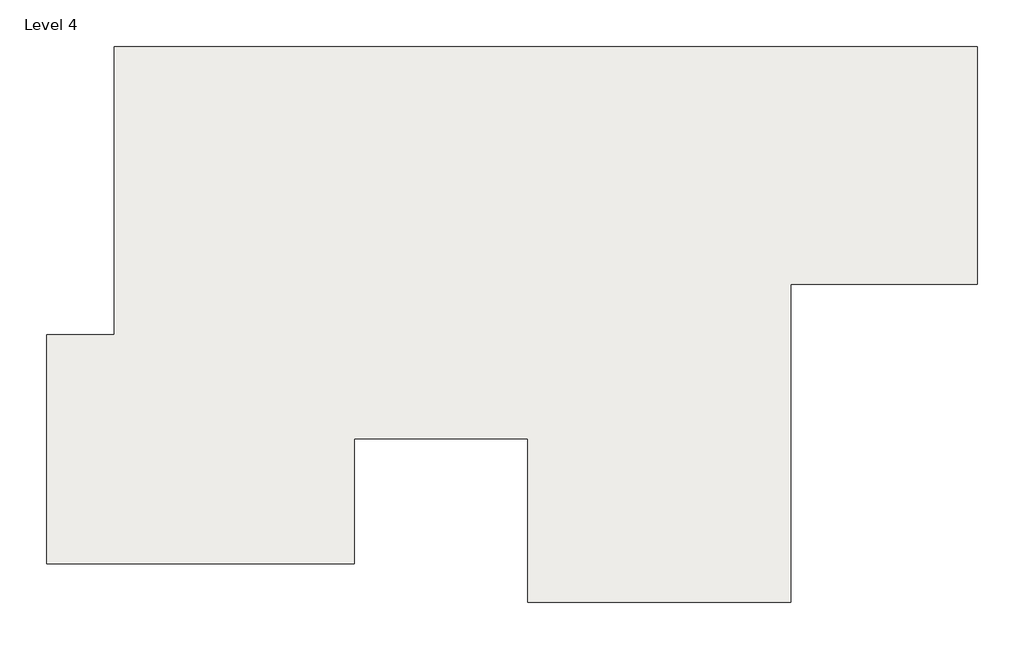
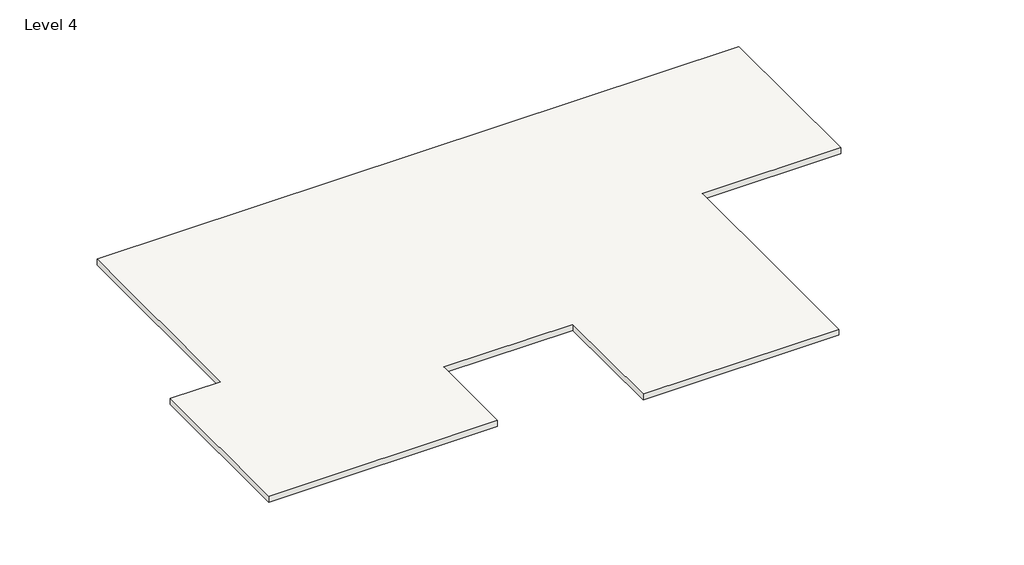
# One storey: 1 roof.
"""IFC4 building model written with IfcOpenShell, lengths in millimetres."""

from ifc_helpers import new_model, si_unit, frame, origin, place, context, project, spatial, polyline, outline, extrude, element, save

model = new_model("IFC4")

# Units and contexts
model_context = context("Model", 3, world=origin())
ifc_project = project(units=[si_unit("LENGTHUNIT", "METRE", prefix="MILLI")], contexts=[model_context])

# Site, building, storey
site = spatial("IfcSite", under=ifc_project)
building = spatial("IfcBuilding", under=site)
storey = spatial("IfcBuildingStorey", under=building, Name="Level 4", Elevation=6248.4)

# Roof
placement = place(None, origin())
element("IfcRoof", 1, ObjectType="6\" roof", at=placement, inside=storey, context=model_context, shape_type="SweptSolid", body=[
    extrude(outline(polyline([(-10562.4981007, 13723.8700124), (4944.2018993, 13723.8700124), (4944.2018993, 9456.6700124), (1591.4018993, 9456.6700124), (1591.4018993, 6300.0267693), (1591.4018993, 3741.6700124), (-3132.9981007, 3741.6700124), (-3132.9981007, 6675.3700124), (-6257.1981007, 6675.3700124), (-6257.1981007, 4427.4700124), (-11781.6981007, 4427.4700124), (-11781.6981007, 8542.2700124), (-10562.4981007, 8542.2700124), (-10562.4981007, 13723.8700124)])), frame((0.0, 0.0, 6705.6), z_axis=(0.0, 0.0, 1.0), x_axis=(1.0, 0.0, 0.0)), (0.0, 0.0, 1.0), 152.4),
])

save(model, "model.ifc")

# Revit data of these elements
# Type "6\" roof"
#   Assembly Code = "B1020"
#   Layers, outside or top first: 0' - 6" no material (function 1)
# Element 1 (IfcRoof, "6\" roof")
#   built-in parameter 1001705 = 22.5 (stored number, unit not read)
#   built-in parameter 1001701 = 1.5 (stored number, unit not read)
#   built-in parameter 1001710 = 33615
#   Phase Created = New Construction
#   Materials on its faces: "Default Roof"
# Materials
#   "Default Roof": colour RGB 88 101 114, transparency 0, Cost = 0
